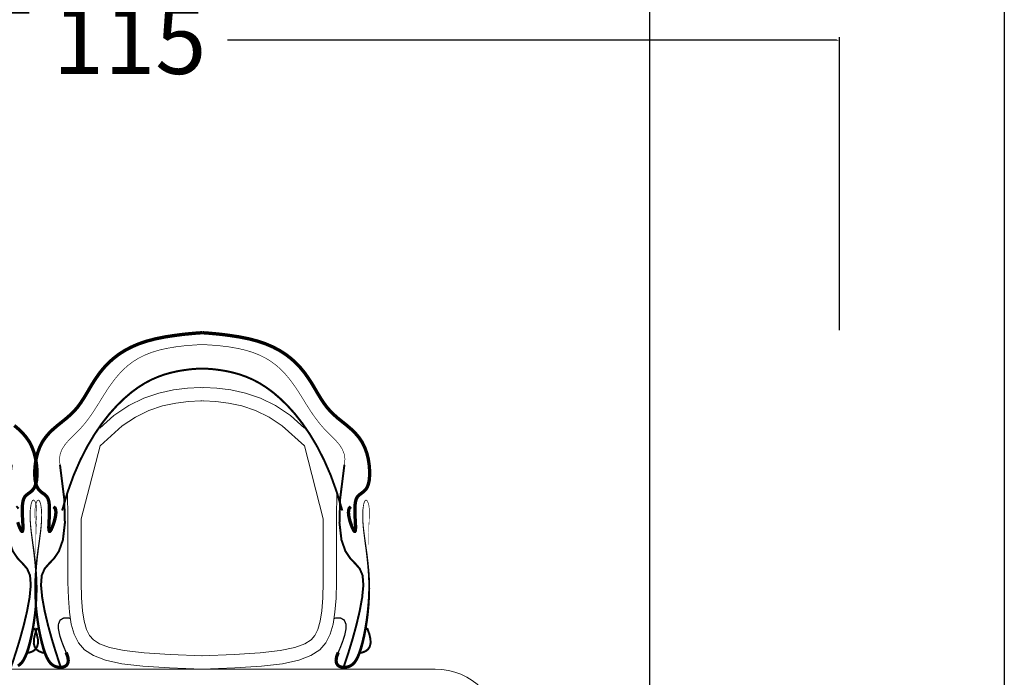
# Model space of a CAD drawing. Units: inches. Extents: x 870 to 1431, y 383 to 1070.
# Tile 7 of 9: x 1171 to 1230, y 718 to 756. Entities that reach past the tile are written whole.
import ezdxf

# ---------------------------------------------------------------- set-up
doc = ezdxf.new("R2010")
doc.units = ezdxf.units.IN
doc.header["$MEASUREMENT"] = 0
doc.layers.add('A-ANNO-DIMS', color=2, linetype='Continuous', lineweight=18)
doc.layers.add('A-FURN', color=8, linetype='Continuous', lineweight=18)
doc.styles.get("Standard").update_dxf_attribs({"font": 'arial.ttf'})
doc.dimstyles.get("Standard").update_dxf_attribs({"dimtxt": 4, "dimasz": 0.18, "dimexe": 0.18, "dimexo": 0.0625, "dimgap": 0.09, "dimtad": 0, "dimtih": 1, "dimtoh": 1, "dimdec": 0, "dimrnd": 6, "dimzin": 0, "dimdsep": 46, "dimlunit": 3, "dimtxsty": 'Standard', "dimcen": 0.09, "dimadec": 0, "dimazin": 0, "dimtfac": 1, "dimtdec": 0, "dimtofl": 0, "dimtmove": 0, "dimatfit": 3, "dimfxl": 1, "dimtolj": 1, "dimtzin": 0, "dimarcsym": 0})

# ---------------------------------------------------------------- blocks, each defined once
blk = doc.blocks.new('ОГ53_на8персон_стол1900х900')
blk.add_line((-850, 279.3), (850, 279.3))
for points, const_width in [([(223.4, 523.4), (221.2, 521.4)], 5), ([(222.7, 500.1), (224.2, 495.7), (225.7, 492), (227, 489.2), (228, 487.3), (228.9, 486.4), (229.6, 486.4), (230.1, 487.3), (230.4, 489.1), (230.6, 491.8), (230.5, 495.4), (230.3, 499.8), (230, 504.9), (229.7, 510.3), (229.6, 516), (229.6, 521.5), (229.9, 526.8), (230.6, 531.5), (231.8, 535.5), (233.5, 538.5), (235.7, 540.8), (238.2, 542.8), (240.8, 544.6), (243.4, 546.7), (245.9, 549.3), (248.1, 552.7), (249.8, 557.2), (251.1, 563.1), (251.7, 570.2), (251.7, 578.1), (251, 586.6), (249.6, 595.4), (247.4, 604.2), (244.3, 612.7), (240.4, 620.6), (235.5, 627.7), (230, 634.2), (223.9, 640.1), (217.5, 645.6)], 5), ([(276.6, 523.4), (278.8, 521.4), (279.9, 518.2), (280.1, 514.2), (279.6, 509.6), (278.6, 504.8), (277.3, 500.1), (275.8, 495.7), (274.3, 492), (273, 489.2), (272, 487.3), (271.1, 486.4), (270.4, 486.4), (269.9, 487.3), (269.6, 489.1), (269.4, 491.8), (269.5, 495.4), (269.7, 499.8), (270, 504.9), (270.3, 510.3), (270.4, 516), (270.4, 521.5), (270.1, 526.8), (269.4, 531.5), (268.2, 535.5), (266.5, 538.5), (264.3, 540.8), (261.8, 542.8), (259.2, 544.6), (256.6, 546.7), (254.1, 549.3), (251.9, 552.7), (250.2, 557.2), (248.9, 563.1), (248.3, 570.2), (248.3, 578.1), (249, 586.6), (250.4, 595.4), (252.6, 604.2), (255.7, 612.7), (259.6, 620.6), (264.5, 627.7), (270, 634.2), (276.1, 640.1), (282.5, 645.6), (289.1, 650.9), (295.7, 656.2), (301.9, 661.7), (307.8, 667.5), (313.1, 673.7), (317.9, 680.3), (322.4, 687.3), (326.8, 694.5), (331.1, 701.9), (335.6, 709.4), (340.5, 716.9), (345.8, 724.4), (351.7, 731.7), (358.3, 738.8), (365.7, 745.6), (373.9, 752), (383.1, 758), (393.3, 763.4), (404.6, 768.3), (417, 772.5), (430.5, 776), (444.6, 778.8), (458.5, 780.9), (471.4, 782.6), (482.8, 783.7), (491.8, 784.5), (497.8, 784.9), (500, 785)], 5), ([(723.4, 523.4), (721.2, 521.4), (720.1, 518.2), (719.9, 514.2), (720.4, 509.6), (721.4, 504.8), (722.7, 500.1), (724.2, 495.7), (725.7, 492), (727, 489.2), (728, 487.3), (728.9, 486.4), (729.6, 486.4), (730.1, 487.3), (730.4, 489.1), (730.6, 491.8), (730.5, 495.4), (730.3, 499.8), (730, 504.9), (729.7, 510.3), (729.6, 516), (729.6, 521.5), (729.9, 526.8), (730.6, 531.5), (731.8, 535.5), (733.5, 538.5), (735.7, 540.8), (738.2, 542.8), (740.8, 544.6), (743.4, 546.7), (745.9, 549.3), (748.1, 552.7), (749.8, 557.2), (751.1, 563.1), (751.7, 570.2), (751.7, 578.1), (751, 586.6), (749.6, 595.4), (747.4, 604.2), (744.3, 612.7), (740.4, 620.6), (735.5, 627.7), (730, 634.2), (723.9, 640.1), (717.5, 645.6), (710.9, 650.9), (704.3, 656.2), (698.1, 661.7), (692.2, 667.5), (686.9, 673.7), (682.1, 680.3), (677.6, 687.3), (673.2, 694.5), (668.9, 701.9), (664.4, 709.4), (659.5, 716.9), (654.2, 724.4), (648.3, 731.7), (641.7, 738.8), (634.3, 745.6), (626.1, 752), (616.9, 758), (606.7, 763.4), (595.4, 768.3), (583, 772.5), (569.5, 776), (555.4, 778.8), (541.5, 780.9), (528.6, 782.6), (517.2, 783.7), (508.2, 784.5), (502.2, 784.9), (500, 785)], 5), ([(286.2, 586.5), (285.4, 595.2), (286.6, 603), (289.5, 610.1), (293.7, 616.6), (298.9, 622.8), (304.7, 628.7), (310.7, 634.6), (316.6, 640.6), (322.1, 646.8), (327.2, 653.3), (332.1, 659.9), (336.7, 666.7), (341.2, 673.7), (345.6, 680.7), (350, 687.9), (354.5, 695), (359.2, 702.2), (364.2, 709.3), (369.5, 716.3), (375.3, 723.1), (381.5, 729.6), (388.3, 735.7), (395.9, 741.4), (404.1, 746.6), (413.3, 751.2), (423.3, 755.2), (434.5, 758.7), (446.7, 761.5), (460.2, 763.8), (475.1, 765.6), (491.4, 766.8), (500, 767.1)], 1), ([(713.8, 586.5), (714.6, 595.2), (713.4, 603), (710.5, 610.1), (706.3, 616.6), (701.1, 622.8), (695.3, 628.7), (689.3, 634.6), (683.4, 640.6), (677.9, 646.8), (672.8, 653.3), (667.9, 659.9), (663.3, 666.7), (658.8, 673.7), (654.4, 680.7), (650, 687.9), (645.5, 695), (640.8, 702.2), (635.8, 709.3), (630.5, 716.3), (624.7, 723.1), (618.5, 729.6), (611.7, 735.7), (604.1, 741.4), (595.9, 746.6), (586.7, 751.2), (576.7, 755.2), (565.5, 758.7), (553.3, 761.5), (539.8, 763.8), (524.9, 765.6), (508.6, 766.8), (500, 767.1)], 1), ([(289.4, 517.6), (297.7, 545.4), (306.8, 570.7), (316.8, 593.6), (327.3, 614.1), (338.2, 632.4), (349.4, 648.7), (360.6, 663), (371.8, 675.4), (382.8, 686.1), (393.5, 695.3), (404, 703), (414.2, 709.4), (424.3, 714.7), (434.1, 718.9), (443.6, 722.3), (453, 724.9), (462.1, 727), (470.7, 728.5), (478.7, 729.6), (485.7, 730.4), (491.6, 730.8), (496.1, 731), (499, 731.1), (500, 731.1)], 3), ([(710.6, 517.6), (702.3, 545.4), (693.2, 570.7), (683.2, 593.6), (672.7, 614.1), (661.8, 632.4), (650.6, 648.7), (639.4, 663), (628.2, 675.4), (617.2, 686.1), (606.5, 695.3), (596, 703), (585.8, 709.4), (575.7, 714.7), (565.9, 718.9), (556.4, 722.3), (547, 724.9), (537.9, 727), (529.3, 728.5), (521.3, 729.6), (514.3, 730.4), (508.4, 730.8), (503.9, 731), (501, 731.1), (500, 731.1)], 3), ([(213.8, 586.5), (207.4, 535.5), (206.4, 498.8), (209.4, 473.4), (215.3, 456.6), (222.6, 445.7), (230.2, 437.8), (236.8, 430.2), (241.2, 420), (242.3, 405.3), (240.5, 386.7), (236.7, 366), (231.6, 344.5), (225.9, 323.8), (220.3, 305.4), (215.6, 291), (212.5, 281.9)], 3), ([(286.2, 586.5), (292.6, 535.5), (293.6, 498.8), (290.6, 473.4), (284.7, 456.6), (277.4, 445.7), (269.8, 437.8), (263.2, 430.2), (258.8, 420), (257.7, 405.3), (259.5, 386.7), (263.3, 366), (268.4, 344.5), (274.1, 323.8), (279.7, 305.4), (284.4, 291), (287.5, 281.9)], 3), ([(713.8, 586.5), (707.4, 535.5), (706.4, 498.8), (709.4, 473.4), (715.3, 456.6), (722.6, 445.7), (730.2, 437.8), (736.8, 430.2), (741.2, 420), (742.3, 405.3), (740.5, 386.7), (736.7, 366), (731.6, 344.5), (725.9, 323.8), (720.3, 305.4), (715.6, 291), (712.5, 281.9)], 3), ([(295.5, 304.2), (292.2, 312), (288.7, 321), (285.7, 330.3), (283.9, 339.3), (284, 347.1), (286.5, 353), (292.2, 356.1), (301.8, 355.7)], 2), ([(704.5, 304.2), (707.8, 312), (711.3, 321), (714.3, 330.3), (716.1, 339.3), (716, 347.1), (713.5, 353), (707.8, 356.1), (698.2, 355.7)], 2), ([(248, 341), (251.3, 331.8), (253, 324.1), (253.1, 317.8), (251.9, 312.9), (249.4, 309), (245.8, 306.2), (241.2, 304.3), (235.7, 303.1)], 3), ([(252, 341), (248.7, 331.8), (247, 324.1), (246.9, 317.8), (248.1, 312.9), (250.6, 309), (254.2, 306.2), (258.8, 304.3), (264.3, 303.1)], 3), ([(748, 341), (751.3, 331.8), (753, 324.1), (753.1, 317.8), (751.9, 312.9), (749.4, 309), (745.8, 306.2), (741.2, 304.3), (735.7, 303.1)], 3)]:
    blk.add_lwpolyline(points, dxfattribs=dict(const_width=const_width))
for points in [[(346, 641.6), (367.4, 660.8), (389.6, 675.6), (412.2, 686.5), (434.8, 694.2), (456.9, 699), (478, 701.6), (497.7, 702.5), (500, 702.4)], [(654, 641.6), (632.6, 660.8), (610.4, 675.6), (587.8, 686.5), (565.2, 694.2), (543.1, 699), (522, 701.6), (502.3, 702.5), (500, 702.4)], [(346.4, 615), (379.7, 644.9), (399.5, 658.2), (419.8, 668), (440.2, 674.9), (460.2, 679.3), (479.6, 681.7), (497.9, 682.5), (499.6, 682.4)], [(653.6, 615), (620.3, 644.9), (600.5, 658.2), (580.2, 668), (559.8, 674.9), (539.8, 679.3), (520.4, 681.7), (502.1, 682.5), (500.4, 682.4)], [(346.4, 615), (318.1, 505.2), (318.1, 469.2), (318, 437.6), (318.1, 410.1), (318.8, 386.6), (320.2, 367), (322.7, 351.1), (326.2, 338.8), (330.6, 329.9), (336.4, 323.3), (345.6, 317.4), (360.5, 311.8), (382.7, 307), (412.9, 303.4), (451.9, 300.9), (500.6, 299.3)], [(653.6, 615), (681.9, 505.2), (681.9, 469.2), (682, 437.6), (681.9, 410.1), (681.2, 386.6), (679.8, 367), (677.3, 351.1), (673.8, 338.8), (669.4, 329.9), (663.6, 323.3), (654.4, 317.4), (639.5, 311.8), (617.3, 307), (587.1, 303.4), (548.1, 300.9), (499.4, 299.3)], [(297.7, 545.4), (298.1, 505.1), (298.1, 469.2), (298, 437.5), (298.1, 409.8), (298.8, 385.6), (300.4, 364.7), (303.2, 346.8), (307.5, 331.5), (313.9, 318.7), (323.2, 308), (336.5, 299.4), (354.9, 292.5), (379.4, 287.3), (411, 283.5), (450.9, 280.9), (500, 279.3)], [(702.3, 545.4), (701.9, 505.1), (701.9, 469.2), (702, 437.5), (701.9, 409.8), (701.2, 385.6), (699.6, 364.7), (696.8, 346.8), (692.5, 331.5), (686.1, 318.7), (676.8, 308), (663.5, 299.4), (645.1, 292.5), (620.6, 287.3), (589, 283.5), (549.1, 280.9), (500, 279.3)]]:
    blk.add_lwpolyline(points)
for points in [[(222.9, 284.1, 4.47, 4.43, 0), (225.9, 286.1, 4.43, 4.38, 0), (228.7, 288.8, 4.38, 4.32, 0), (231.3, 292.5, 4.32, 4.25, 0), (233.8, 297.3, 4.25, 4.17, 0), (236.3, 303.2, 4.17, 4.07, 0), (238.7, 310.4, 4.07, 3.95, 0), (241, 318.9, 3.95, 3.82, 0), (243.3, 328.7, 3.82, 3.68, 0), (245.4, 339.4, 3.68, 3.53, 0), (247.2, 350.9, 3.53, 3.37, 0), (248.8, 363, 3.37, 3.21, 0), (250, 375.5, 3.21, 3.05, 0), (250.8, 388.2, 3.05, 2.88, 0), (251.1, 400.7, 2.88, 2.72, 0), (250.9, 413.1, 2.72, 2.57, 0), (250.2, 425.1, 2.57, 2.41, 0), (249.2, 436.7, 2.41, 2.27, 0), (248, 447.8, 2.27, 2.13, 0), (246.7, 458.3, 2.13, 2, 0), (245.3, 468.2, 2, 1.88, 0), (244.1, 477.3, 1.88, 1.78, 0), (243, 485.6, 1.78, 1.68, 0), (242.2, 493.1, 1.68, 1.59, 0), (241.7, 499.6, 1.59, 1.52, 0), (241.4, 505.4, 1.52, 1.45, 0), (241.3, 510.5, 1.45, 1.4, 0), (241.4, 514.9, 1.4, 1.35, 0), (241.6, 518.7, 1.35, 1.3, 0), (242, 521.9, 1.3, 1.27, 0), (242.4, 524.7, 1.27, 1.24, 0), (242.8, 527, 1.24, 1.21, 0), (243.3, 528.8, 1.21, 1.19, 0), (243.8, 530.3, 1.19, 1.18, 0), (244.3, 531.5, 1.18, 1.16, 0), (244.8, 532.3, 1.16, 1.15, 0), (245.3, 532.9, 1.15, 1.14, 0), (245.8, 533.2, 1.14, 1.14, 0), (246.3, 533.3, 1.14, 1.13, 0), (246.8, 533.2, 1.13, 1.12, 0), (247.3, 533, 1.12, 1.12, 0), (247.8, 532.5, 1.12, 1.11, 0), (248.3, 531.9, 1.11, 1.09, 0), (248.7, 531.1, 1.09, 1.08, 0), (249.1, 530.2, 1.08, 1.07, 0), (249.5, 529.1, 1.07, 1.05, 0), (249.9, 527.9, 1.05, 1.03, 0), (250.3, 526.5, 1.03, 1.01, 0), (250.6, 524.9, 1.01, 0.986, 0), (250.9, 523.1, 0.986, 0.959, 0), (251.1, 521, 0.959, 0.926, 0), (251.3, 518.5, 0.926, 0.889, 0), (251.4, 515.7, 0.889, 0.846, 0), (251.4, 512.3, 0.846, 0.796, 0), (251.3, 508.5, 0.796, 0.738, 0), (251.1, 504, 0.738, 0.672, 0), (250.8, 498.9, 0.672, 0.595, 0), (250.6, 493, 0.595, 0.506, 0), (250.3, 486.1, 0.506, 0.404, 0), (250.1, 478.2, 0.404, 0.286, 0), (249.9, 469.2, 0.286, 0.152, 0), (249.9, 458.8, 0.152, 0, 0), (250, 447.1, 0, 0, 0)], [(295.5, 304.2, 5, 4.91, 0), (298, 297.4, 4.91, 4.84, 0), (298.7, 292.1, 4.84, 4.78, 0), (298.1, 288.1, 4.78, 4.74, 0), (296.3, 285.1, 4.74, 4.7, 0), (293.7, 283.2, 4.7, 4.65, 0), (290.6, 282.2, 4.65, 4.61, 0), (287.1, 281.8, 4.61, 4.56, 0), (283.5, 282.1, 4.56, 4.52, 0), (280.2, 282.8, 4.52, 4.47, 0), (277.1, 284.1, 4.47, 4.43, 0), (274.1, 286.1, 4.43, 4.38, 0), (271.3, 288.8, 4.38, 4.32, 0), (268.7, 292.5, 4.32, 4.25, 0), (266.2, 297.3, 4.25, 4.17, 0), (263.7, 303.2, 4.17, 4.07, 0), (261.3, 310.4, 4.07, 3.95, 0), (259, 318.9, 3.95, 3.82, 0), (256.7, 328.7, 3.82, 3.68, 0), (254.6, 339.4, 3.68, 3.53, 0), (252.8, 350.9, 3.53, 3.37, 0), (251.2, 363, 3.37, 3.21, 0), (250, 375.5, 3.21, 3.05, 0), (249.2, 388.2, 3.05, 2.88, 0), (248.9, 400.7, 2.88, 2.72, 0), (249.1, 413.1, 2.72, 2.57, 0), (249.8, 425.1, 2.57, 2.41, 0), (250.8, 436.7, 2.41, 2.27, 0), (252, 447.8, 2.27, 2.13, 0), (253.3, 458.3, 2.13, 2, 0), (254.7, 468.2, 2, 1.88, 0), (255.9, 477.3, 1.88, 1.78, 0), (257, 485.6, 1.78, 1.68, 0), (257.8, 493.1, 1.68, 1.59, 0), (258.3, 499.6, 1.59, 1.52, 0), (258.6, 505.4, 1.52, 1.45, 0), (258.7, 510.5, 1.45, 1.4, 0), (258.6, 514.9, 1.4, 1.35, 0), (258.4, 518.7, 1.35, 1.3, 0), (258, 521.9, 1.3, 1.27, 0), (257.6, 524.7, 1.27, 1.24, 0), (257.2, 527, 1.24, 1.21, 0), (256.7, 528.8, 1.21, 1.19, 0), (256.2, 530.3, 1.19, 1.18, 0), (255.7, 531.5, 1.18, 1.16, 0), (255.2, 532.3, 1.16, 1.15, 0), (254.7, 532.9, 1.15, 1.14, 0), (254.2, 533.2, 1.14, 1.14, 0), (253.7, 533.3, 1.14, 1.13, 0), (253.2, 533.2, 1.13, 1.12, 0), (252.7, 533, 1.12, 1.12, 0), (252.2, 532.5, 1.12, 1.11, 0), (251.7, 531.9, 1.11, 1.09, 0), (251.3, 531.1, 1.09, 1.08, 0), (250.9, 530.2, 1.08, 1.07, 0), (250.5, 529.1, 1.07, 1.05, 0), (250.1, 527.9, 1.05, 1.03, 0), (249.7, 526.5, 1.03, 1.01, 0), (249.4, 524.9, 1.01, 0.986, 0), (249.1, 523.1, 0.986, 0.959, 0), (248.9, 521, 0.959, 0.926, 0), (248.7, 518.5, 0.926, 0.889, 0), (248.6, 515.7, 0.889, 0.846, 0), (248.6, 512.3, 0.846, 0.796, 0), (248.7, 508.5, 0.796, 0.738, 0), (248.9, 504, 0.738, 0.672, 0), (249.2, 498.9, 0.672, 0.595, 0), (249.4, 493, 0.595, 0.506, 0), (249.7, 486.1, 0.506, 0.404, 0), (249.9, 478.2, 0.404, 0.286, 0), (250.1, 469.2, 0.286, 0.152, 0), (250.1, 458.8, 0.152, 0, 0), (250, 447.1, 0, 0, 0)], [(704.5, 304.2, 5, 4.91, 0), (702, 297.4, 4.91, 4.84, 0), (701.3, 292.1, 4.84, 4.78, 0), (701.9, 288.1, 4.78, 4.74, 0), (703.7, 285.1, 4.74, 4.7, 0), (706.3, 283.2, 4.7, 4.65, 0), (709.4, 282.2, 4.65, 4.61, 0), (712.9, 281.8, 4.61, 4.56, 0), (716.5, 282.1, 4.56, 4.52, 0), (719.8, 282.8, 4.52, 4.47, 0), (722.9, 284.1, 4.47, 4.43, 0), (725.9, 286.1, 4.43, 4.38, 0), (728.7, 288.8, 4.38, 4.32, 0), (731.3, 292.5, 4.32, 4.25, 0), (733.8, 297.3, 4.25, 4.17, 0), (736.3, 303.2, 4.17, 4.07, 0), (738.7, 310.4, 4.07, 3.95, 0), (741, 318.9, 3.95, 3.82, 0), (743.3, 328.7, 3.82, 3.68, 0), (745.4, 339.4, 3.68, 3.53, 0), (747.2, 350.9, 3.53, 3.37, 0), (748.8, 363, 3.37, 3.21, 0), (750, 375.5, 3.21, 3.05, 0), (750.8, 388.2, 3.05, 2.88, 0), (751.1, 400.7, 2.88, 2.72, 0), (750.9, 413.1, 2.72, 2.57, 0), (750.2, 425.1, 2.57, 2.41, 0), (749.2, 436.7, 2.41, 2.27, 0), (748, 447.8, 2.27, 2.13, 0), (746.7, 458.3, 2.13, 2, 0), (745.3, 468.2, 2, 1.88, 0), (744.1, 477.3, 1.88, 1.78, 0), (743, 485.6, 1.78, 1.68, 0), (742.2, 493.1, 1.68, 1.59, 0), (741.7, 499.6, 1.59, 1.52, 0), (741.4, 505.4, 1.52, 1.45, 0), (741.3, 510.5, 1.45, 1.4, 0), (741.4, 514.9, 1.4, 1.35, 0), (741.6, 518.7, 1.35, 1.3, 0), (742, 521.9, 1.3, 1.27, 0), (742.4, 524.7, 1.27, 1.24, 0), (742.8, 527, 1.24, 1.21, 0), (743.3, 528.8, 1.21, 1.19, 0), (743.8, 530.3, 1.19, 1.18, 0), (744.3, 531.5, 1.18, 1.16, 0), (744.8, 532.3, 1.16, 1.15, 0), (745.3, 532.9, 1.15, 1.14, 0), (745.8, 533.2, 1.14, 1.14, 0), (746.3, 533.3, 1.14, 1.13, 0), (746.8, 533.2, 1.13, 1.12, 0), (747.3, 533, 1.12, 1.12, 0), (747.8, 532.5, 1.12, 1.11, 0), (748.3, 531.9, 1.11, 1.09, 0), (748.7, 531.1, 1.09, 1.08, 0), (749.1, 530.2, 1.08, 1.07, 0), (749.5, 529.1, 1.07, 1.05, 0), (749.9, 527.9, 1.05, 1.03, 0), (750.3, 526.5, 1.03, 1.01, 0), (750.6, 524.9, 1.01, 0.986, 0), (750.9, 523.1, 0.986, 0.959, 0), (751.1, 521, 0.959, 0.926, 0), (751.3, 518.5, 0.926, 0.889, 0), (751.4, 515.7, 0.889, 0.846, 0), (751.4, 512.3, 0.846, 0.796, 0), (751.3, 508.5, 0.796, 0.738, 0), (751.1, 504, 0.738, 0.672, 0), (750.8, 498.9, 0.672, 0.595, 0), (750.6, 493, 0.595, 0.506, 0), (750.3, 486.1, 0.506, 0.404, 0), (750.1, 478.2, 0.404, 0.286, 0), (749.9, 469.2, 0.286, 0.152, 0), (749.9, 458.8, 0.152, 0, 0), (750, 447.1, 0, 0, 0)]]:
    blk.add_lwpolyline(points, format="xyseb")
blk.add_arc((850, 179.3), 100, 0, 90)
blk = doc.blocks.new('*D123')
at = {"layer": 'A-ANNO-DIMS', "color": 0, "lineweight": -2, "transparency": 16777216}
for p, q in [((1104.966, 738.101), (1104.966, 755.441)), ((1105.146, 755.261), (1141.184, 755.261)), ((1219.601, 755.261), (1183.563, 755.261)), ((1219.781, 738.101), (1219.781, 755.441))]:
    blk.add_line(p, q, dxfattribs=at)
at = {"layer": 'A-ANNO-DIMS', "color": 0, "transparency": 16777216}
for points in [[(1105.146, 755.291), (1105.146, 755.231), (1104.966, 755.261)], [(1219.601, 755.291), (1219.601, 755.231), (1219.781, 755.261)]]:
    blk.add_solid(points, dxfattribs=at)
at = {"layer": 'Defpoints', "color": 0, "transparency": 16777216}
for p in [(1219.781, 755.261), (1104.966, 738.039), (1219.781, 738.039)]:
    blk.add_point(p, dxfattribs=at)
at = {"layer": 'A-ANNO-DIMS', "color": 0, "transparency": 16777216, "insert": (1162.373, 755.261), "char_height": 4, "attachment_point": 5}
blk.add_mtext('\\A1;DINING SET 115', dxfattribs=at)
blk = doc.blocks.new('*D136')
at = {"layer": 'A-ANNO-DIMS', "color": 0, "lineweight": -2, "transparency": 16777216}
for p, q in [((1208.533, 986.128), (1208.533, 385.26)), ((1229.533, 986.128), (1229.533, 385.26)), ((1208.713, 385.44), (1216.43, 385.44)), ((1229.353, 385.44), (1221.636, 385.44))]:
    blk.add_line(p, q, dxfattribs=at)
at = {"layer": 'A-ANNO-DIMS', "color": 0, "transparency": 16777216}
for points in [[(1208.713, 385.47), (1208.713, 385.41), (1208.533, 385.44)], [(1229.353, 385.47), (1229.353, 385.41), (1229.533, 385.44)]]:
    blk.add_solid(points, dxfattribs=at)
at = {"layer": 'Defpoints', "color": 0, "transparency": 16777216}
for p in [(1208.533, 986.191), (1229.533, 986.191), (1229.533, 385.44)]:
    blk.add_point(p, dxfattribs=at)
at = {"layer": 'A-ANNO-DIMS', "color": 0, "transparency": 16777216, "insert": (1219.033, 385.44), "char_height": 4, "attachment_point": 5}
blk.add_mtext('\\A1;21', dxfattribs=at)

msp = doc.modelspace()

# ---------------------------------------------------------------- block references
at = {"layer": 'A-FURN', "xscale": 0.0393700787401575, "yscale": 0.0393700787401575, "zscale": 0.0393700787401575}
msp.add_blockref('ОГ53_на8персон_стол1900х900', (1162.3732, 707.036), dxfattribs=at)

# ---------------------------------------------------------------- dimensions: what is measured, and where the dimension line sits
at = {"layer": 'A-ANNO-DIMS'}
dim = msp.add_linear_dim(base=(1229.5328, 385.44), p1=(1208.5328, 986.1907), p2=(1229.5328, 986.1907), dimstyle='Standard', override={"dimdec": 0, "dimlfac": 1, "dimrnd": 0, "dimzin": 0, "dimdsep": 46, "dimlunit": 2}, dxfattribs=at)
dim.commit()
dim.dimension.update_dxf_attribs({"geometry": '*D136', "text_midpoint": (1219.0328, 385.44)})
dim = msp.add_linear_dim(base=(1219.7806, 755.2609), p1=(1104.9659, 738.0387), p2=(1219.7806, 738.0387), text='DINING SET <>', dimstyle='Standard', override={"dimdec": 0, "dimlfac": 1, "dimrnd": 0, "dimzin": 0, "dimdsep": 46, "dimlunit": 2}, dxfattribs=at)
dim.commit()
dim.dimension.update_dxf_attribs({"geometry": '*D123', "text_midpoint": (1162.3732, 755.2609)})

doc.saveas('drawing.dxf')
